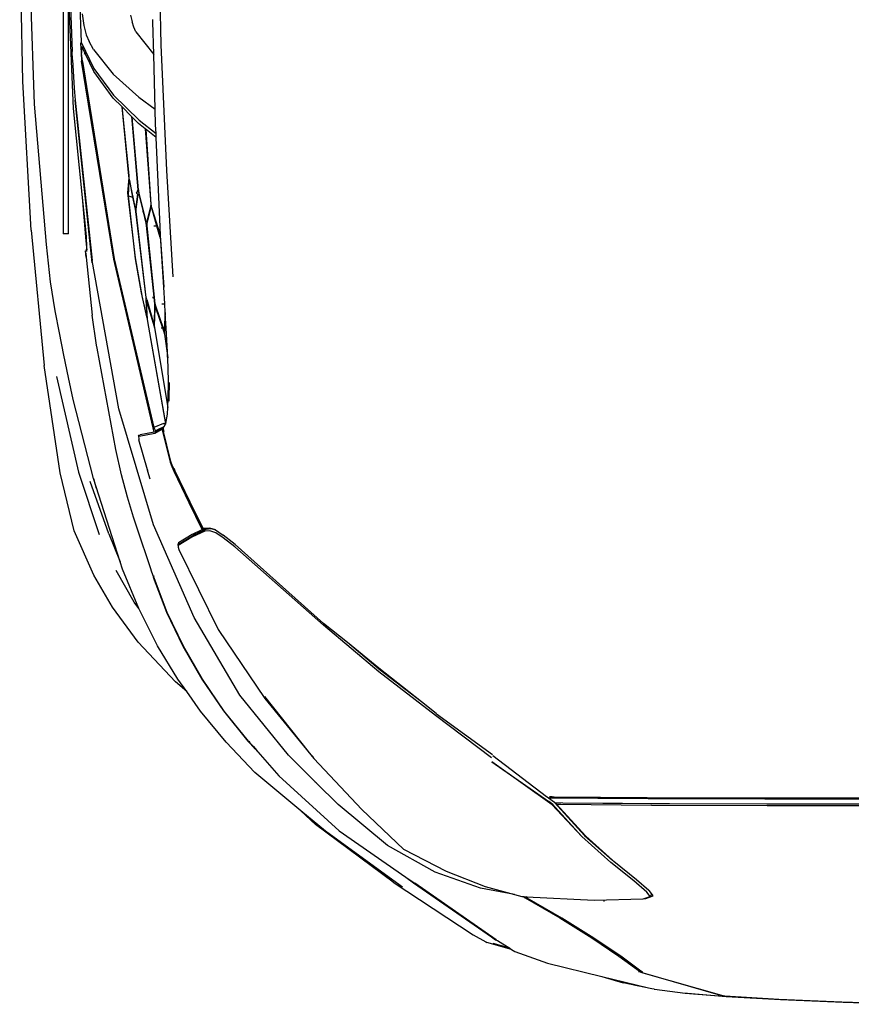
# Model space of a CAD drawing. Units: inches. Extents: x 22042254 to 25404563, y 17568978 to 17626777.
# Tile 10 of 45: x 22042340.5158 to 22042340.9417, y 17568977.6618 to 17568978.1657. Entities that reach past the tile are written whole.
import ezdxf

# ---------------------------------------------------------------- set-up
doc = ezdxf.new("R2010")
doc.units = ezdxf.units.IN
doc.header["$MEASUREMENT"] = 0
doc.layers.add('A-SITE-VEHI', color=8, linetype='Continuous', lineweight=18)
doc.layers.add('Edges', color=250, linetype='Continuous')

# ---------------------------------------------------------------- blocks, each defined once
blk = doc.blocks.new('Nissan Qashqai pl')
at = {"layer": 'Edges'}
for p, q in [((8.01597, 12.81888), (7.96577, 12.81715)), ((7.96683, 12.81735), (8.01677, 12.81906)), ((7.86763, 12.81233), (7.79979, 12.79282)), ((7.80119, 12.79291), (7.86805, 12.81214)), ((7.83626, 12.80972), (7.86763, 12.81233)), ((7.83812, 12.80996), (7.86997, 12.81262)), ((7.86763, 12.81233), (7.86805, 12.81214)), ((7.86903, 12.81242), (7.86805, 12.81214)), ((7.91369, 12.81497), (7.86903, 12.81242)), ((7.86997, 12.81262), (7.91514, 12.8152)), ((7.96577, 12.81715), (7.91369, 12.81497)), ((7.91514, 12.8152), (7.96683, 12.81735)), ((7.7673, 12.79611), (7.80585, 12.80552)), ((7.80866, 12.80621), (7.78484, 12.80117)), ((7.79357, 12.80288), (7.79772, 12.80375)), ((7.81062, 12.80645), (7.80866, 12.80621)), ((7.81062, 12.80645), (7.81073, 12.80648)), ((7.81073, 12.80648), (7.83626, 12.80972)), ((7.83626, 12.80972), (7.83812, 12.80996)), ((7.72226, 12.78511), (7.7673, 12.79611)), ((7.7673, 12.79611), (7.78484, 12.80117)), ((7.78354, 12.80068), (7.78351, 12.80067)), ((7.78647, 12.80131), (7.78656, 12.80134)), ((7.78138, 12.77913), (7.79909, 12.7923)), ((7.79842, 12.79085), (7.78285, 12.7793)), ((7.79759, 12.79204), (7.79909, 12.7923)), ((7.80074, 12.79258), (7.79842, 12.79085)), ((7.79909, 12.7923), (7.79979, 12.79282)), ((7.79952, 12.79237), (7.80074, 12.79258)), ((7.80119, 12.79291), (7.80074, 12.79258)), ((7.69527, 12.77535), (7.72226, 12.78511)), ((7.75906, 12.76414), (7.78138, 12.77913)), ((7.78285, 12.7793), (7.76061, 12.76436)), ((7.6926, 12.77369), (7.67207, 12.76794)), ((7.69111, 12.77277), (7.67743, 12.76878)), ((7.68089, 12.76644), (7.69111, 12.77277)), ((7.69111, 12.77277), (7.6926, 12.77369)), ((7.6926, 12.77369), (7.69527, 12.77535)), ((7.59458, 12.71797), (7.66077, 12.76166)), ((7.61132, 12.71859), (7.67585, 12.76329)), ((7.67993, 12.76585), (7.61247, 12.71901)), ((7.66077, 12.76166), (7.67122, 12.76746)), ((7.67122, 12.76746), (7.67207, 12.76794)), ((7.67585, 12.76329), (7.67933, 12.76572)), ((7.67933, 12.76572), (7.68018, 12.766)), ((7.67993, 12.76585), (7.68018, 12.766)), ((7.68018, 12.766), (7.68089, 12.76644)), ((7.73247, 12.74757), (7.75906, 12.76414)), ((7.76061, 12.76436), (7.73411, 12.74784)), ((7.70382, 12.731), (7.73247, 12.74757)), ((7.73411, 12.74784), (7.70559, 12.73137)), ((7.69488, 12.72832), (7.70101, 12.73001)), ((7.70101, 12.73001), (7.70235, 12.73008)), ((7.70235, 12.73008), (7.70382, 12.731)), ((7.70235, 12.73008), (7.70343, 12.73013)), ((7.70559, 12.73137), (7.70343, 12.73013)), ((7.70343, 12.73013), (7.70481, 12.7302)), ((7.70481, 12.7302), (7.76082, 12.73292)), ((7.70579, 12.73076), (7.70481, 12.7302)), ((7.76082, 12.73292), (7.80143, 12.73178)), ((7.76878, 12.73282), (7.76885, 12.73399)), ((7.80143, 12.73178), (7.80216, 12.73156)), ((7.80216, 12.73156), (7.80372, 12.73151)), ((7.80216, 12.73156), (7.80721, 12.73004)), ((7.80372, 12.73151), (7.80956, 12.72941)), ((7.80721, 12.73004), (7.80447, 12.72626)), ((7.80956, 12.72941), (7.80665, 12.72539)), ((7.80721, 12.73004), (7.80867, 12.72831)), ((7.60245, 12.72211), (7.53868, 12.67594)), ((7.66697, 12.723), (7.62951, 12.70974)), ((7.63858, 12.70891), (7.67084, 12.72167)), ((7.69488, 12.72832), (7.66697, 12.723)), ((7.67084, 12.72167), (7.69488, 12.72832)), ((7.80447, 12.72626), (7.79381, 12.71706)), ((7.80619, 12.725), (7.79586, 12.71608)), ((7.80619, 12.725), (7.80867, 12.72831)), ((7.80665, 12.72539), (7.80619, 12.725)), ((7.59458, 12.71797), (7.53043, 12.67044)), ((7.55011, 12.67573), (7.60515, 12.71393)), ((7.60515, 12.71393), (7.61132, 12.71859)), ((7.60515, 12.71393), (7.61111, 12.71807)), ((7.61183, 12.71862), (7.61111, 12.71807)), ((7.61247, 12.71901), (7.61183, 12.71862)), ((7.79381, 12.71706), (7.77477, 12.70185)), ((7.79586, 12.71608), (7.77724, 12.70105)), ((7.62951, 12.70974), (7.58999, 12.68766)), ((7.60319, 12.69082), (7.63858, 12.70891)), ((7.77477, 12.70185), (7.75074, 12.68033)), ((7.75301, 12.67941), (7.77596, 12.69989)), ((7.77596, 12.69989), (7.75388, 12.67998)), ((7.77724, 12.70105), (7.77596, 12.69989)), ((7.56866, 12.65792), (7.60319, 12.69082)), ((7.58999, 12.68766), (7.5492, 12.654)), ((7.72614, 12.65431), (7.75074, 12.68033)), ((7.75074, 12.68033), (7.72856, 12.65607)), ((7.55011, 12.67573), (7.50008, 12.63025)), ((7.53868, 12.67594), (7.5184, 12.65911)), ((7.75301, 12.67941), (7.72807, 12.65235)), ((7.75388, 12.67998), (7.73238, 12.65652)), ((7.5184, 12.65911), (7.53043, 12.67044)), ((7.5184, 12.65911), (7.48015, 12.62736)), ((7.52891, 12.61585), (7.56866, 12.65792)), ((7.72856, 12.65607), (7.72667, 12.65393)), ((7.73238, 12.65652), (7.72986, 12.65372)), ((7.5492, 12.654), (7.53101, 12.63591)), ((7.72614, 12.65431), (7.67617, 12.61859)), ((7.67617, 12.61859), (7.72327, 12.65136)), ((7.7215, 12.64734), (7.72214, 12.64782)), ((7.72318, 12.64862), (7.72214, 12.64782)), ((7.72807, 12.65235), (7.72318, 12.64862)), ((7.72455, 12.64863), (7.72318, 12.64862)), ((7.72667, 12.65393), (7.72327, 12.65136)), ((7.72606, 12.64765), (7.72382, 12.64759)), ((7.72942, 12.64868), (7.72455, 12.64863)), ((7.72785, 12.6477), (7.72606, 12.64765)), ((7.80482, 12.64828), (7.72785, 12.6477)), ((7.72986, 12.65372), (7.72807, 12.65235)), ((7.72807, 12.65235), (7.73491, 12.65241)), ((7.73098, 12.64869), (7.72942, 12.64868)), ((7.72986, 12.65372), (7.73345, 12.65375)), ((7.76399, 12.64888), (7.73098, 12.64869)), ((7.73345, 12.65375), (7.80829, 12.65437)), ((7.73491, 12.65241), (7.76799, 12.65269)), ((7.76622, 12.64889), (7.76399, 12.64888)), ((7.78115, 12.64897), (7.76622, 12.64889)), ((7.76799, 12.65269), (7.76925, 12.6527)), ((7.76925, 12.6527), (7.78439, 12.65283)), ((7.78224, 12.64898), (7.78115, 12.64897)), ((7.80566, 12.64911), (7.78224, 12.64898)), ((7.78439, 12.65283), (7.80777, 12.65303)), ((7.90142, 12.64867), (7.80482, 12.64828)), ((7.82329, 12.64918), (7.80566, 12.64911)), ((7.80777, 12.65303), (7.82329, 12.65309)), ((7.80829, 12.65437), (7.90396, 12.65472)), ((7.82329, 12.65309), (7.90357, 12.65342)), ((7.90204, 12.64948), (7.82329, 12.64918)), ((8.02732, 12.64849), (7.90142, 12.64867)), ((8.02749, 12.64934), (7.90204, 12.64948)), ((7.90357, 12.65342), (8.0275, 12.6533)), ((7.90396, 12.65472), (8.02759, 12.65454)), ((7.67714, 12.61347), (7.7215, 12.64734)), ((7.53101, 12.63591), (7.50805, 12.61306)), ((7.53101, 12.63591), (7.53009, 12.6353)), ((7.48015, 12.62736), (7.45654, 12.6023)), ((7.48274, 12.61035), (7.50008, 12.63025)), ((7.48836, 12.56635), (7.52891, 12.61585)), ((7.67598, 12.61523), (7.6296, 12.58026)), ((7.50805, 12.61306), (7.46788, 12.56344)), ((7.47438, 12.60148), (7.48041, 12.60787)), ((7.48041, 12.60787), (7.47799, 12.6049)), ((7.47901, 12.60607), (7.4815, 12.60892)), ((7.47901, 12.60607), (7.48009, 12.6074)), ((7.48009, 12.6074), (7.48041, 12.60787)), ((7.48041, 12.60787), (7.48043, 12.60789)), ((7.48043, 12.60789), (7.48069, 12.60817)), ((7.48069, 12.60817), (7.48214, 12.60971)), ((7.4815, 12.60892), (7.48214, 12.60971)), ((7.48214, 12.60971), (7.48274, 12.61035)), ((7.48817, 12.5645), (7.52431, 12.61007)), ((7.52431, 12.61007), (7.52857, 12.61458)), ((7.67691, 12.61295), (7.63059, 12.57913)), ((7.45654, 12.6023), (7.4354, 12.57664)), ((7.45423, 12.57648), (7.47438, 12.60148)), ((7.47504, 12.60161), (7.45491, 12.57668)), ((7.47616, 12.6028), (7.47504, 12.60161)), ((7.47515, 12.60164), (7.47616, 12.6028)), ((7.47616, 12.6028), (7.47799, 12.6049)), ((7.47799, 12.6049), (7.47901, 12.60607)), ((7.4354, 12.57664), (7.42386, 12.56045)), ((7.43626, 12.55019), (7.45423, 12.57648)), ((7.45491, 12.57668), (7.4369, 12.55039)), ((7.6296, 12.58026), (7.58274, 12.54411)), ((7.63007, 12.57872), (7.61803, 12.56913)), ((7.63059, 12.57913), (7.63007, 12.57872)), ((7.44978, 12.50928), (7.48836, 12.56635)), ((7.61803, 12.56913), (7.58288, 12.54113)), ((7.61803, 12.56913), (7.58398, 12.54289)), ((7.42386, 12.56045), (7.41469, 12.55237)), ((7.42386, 12.56045), (7.41661, 12.55027)), ((7.46788, 12.56344), (7.43015, 12.49926)), ((7.41469, 12.55237), (7.38367, 12.51969)), ((7.41661, 12.55027), (7.39973, 12.5227)), ((7.42053, 12.52292), (7.43626, 12.55019)), ((7.4369, 12.55039), (7.42115, 12.52316)), ((7.58274, 12.54411), (7.53689, 12.50568)), ((7.58398, 12.54289), (7.55683, 12.52012)), ((7.58288, 12.54113), (7.55683, 12.52012)), ((7.38367, 12.51969), (7.36237, 12.49067)), ((7.39973, 12.5227), (7.38446, 12.49246)), ((7.40715, 12.49483), (7.42053, 12.52292)), ((7.42115, 12.52316), (7.40781, 12.49514)), ((7.55683, 12.52012), (7.53708, 12.50419)), ((7.41723, 12.44309), (7.44978, 12.50928)), ((7.53689, 12.50568), (7.46355, 12.44079)), ((7.46382, 12.43903), (7.53708, 12.50419)), ((7.39621, 12.46602), (7.40715, 12.49483)), ((7.43015, 12.49926), (7.39627, 12.4227)), ((7.40781, 12.49514), (7.39687, 12.46646)), ((7.36237, 12.49067), (7.34698, 12.4644)), ((7.38053, 12.48658), (7.36552, 12.46044)), ((7.38426, 12.49197), (7.37074, 12.45925)), ((7.38426, 12.49197), (7.38053, 12.48658)), ((7.38446, 12.49246), (7.38426, 12.49197)), ((7.34698, 12.4644), (7.3309, 12.42757)), ((7.39513, 12.46199), (7.39379, 12.45826)), ((7.39648, 12.46548), (7.39513, 12.46199)), ((7.39648, 12.46548), (7.39621, 12.46602)), ((7.39687, 12.46646), (7.39648, 12.46548)), ((7.39676, 12.46492), (7.39668, 12.46506)), ((7.3688, 12.45323), (7.34671, 12.38455)), ((7.35959, 12.43024), (7.3688, 12.45323)), ((7.37074, 12.45925), (7.3688, 12.45323)), ((7.39247, 12.45422), (7.38454, 12.43058)), ((7.39379, 12.45826), (7.39247, 12.45422)), ((7.41665, 12.43928), (7.41687, 12.44057)), ((7.41665, 12.43928), (7.41716, 12.43948)), ((7.41697, 12.43768), (7.41665, 12.43928)), ((7.41686, 12.44121), (7.41723, 12.44309)), ((7.41687, 12.44057), (7.41686, 12.44121)), ((7.41687, 12.44057), (7.41717, 12.44232)), ((7.41689, 12.43978), (7.41687, 12.44057)), ((7.42821, 12.43284), (7.41689, 12.43978)), ((7.41716, 12.43948), (7.41689, 12.43978)), ((7.42833, 12.4307), (7.41697, 12.43768)), ((7.4183, 12.4382), (7.41716, 12.43948)), ((7.41717, 12.44232), (7.41744, 12.44287)), ((7.41747, 12.44292), (7.41744, 12.44287)), ((7.4183, 12.4382), (7.42961, 12.43124)), ((7.46355, 12.44079), (7.4541, 12.43335)), ((7.46382, 12.43903), (7.45415, 12.43132)), ((7.33449, 12.37926), (7.3514, 12.43082)), ((7.35959, 12.43024), (7.34401, 12.38695)), ((7.38454, 12.43058), (7.37986, 12.41639)), ((7.43873, 12.42797), (7.42821, 12.43284)), ((7.43587, 12.42718), (7.42833, 12.4307)), ((7.43832, 12.42716), (7.42961, 12.43124)), ((7.44309, 12.42761), (7.43873, 12.42797)), ((7.44789, 12.42929), (7.44309, 12.42761)), ((7.44771, 12.42699), (7.45415, 12.43132)), ((7.4541, 12.43335), (7.44789, 12.42929)), ((7.3309, 12.42757), (7.31925, 12.37966)), ((7.39627, 12.4227), (7.36761, 12.32692)), ((7.42553, 12.40435), (7.43673, 12.42678)), ((7.43648, 12.4235), (7.42672, 12.4041)), ((7.43673, 12.42678), (7.43587, 12.42718)), ((7.43651, 12.42353), (7.43648, 12.4235)), ((7.43782, 12.42614), (7.43651, 12.42353)), ((7.43673, 12.42678), (7.43832, 12.42716)), ((7.43787, 12.42625), (7.43782, 12.42614)), ((7.43787, 12.42625), (7.43832, 12.42716)), ((7.43787, 12.42625), (7.4389, 12.42689)), ((7.43844, 12.42599), (7.43787, 12.42625)), ((7.43844, 12.42599), (7.43799, 12.42508)), ((7.43832, 12.42716), (7.4389, 12.42689)), ((7.4389, 12.42689), (7.43844, 12.42599)), ((7.43873, 12.42586), (7.43844, 12.42599)), ((7.44298, 12.42535), (7.43873, 12.42586)), ((7.44004, 12.42635), (7.4389, 12.42689)), ((7.44004, 12.42635), (7.44418, 12.42585)), ((7.44771, 12.42699), (7.44298, 12.42535)), ((7.44418, 12.42585), (7.44771, 12.42699)), ((7.37986, 12.41639), (7.375, 12.39997)), ((7.41315, 12.3783), (7.42553, 12.40435)), ((7.42672, 12.4041), (7.41393, 12.37779)), ((7.375, 12.39997), (7.36995, 12.3813)), ((7.34671, 12.38455), (7.34891, 12.39245)), ((7.31925, 12.37966), (7.3059, 12.29098)), ((7.31612, 12.30008), (7.33449, 12.37926)), ((7.34671, 12.38455), (7.32996, 12.31924)), ((7.36995, 12.3813), (7.36534, 12.36039)), ((7.39248, 12.38132), (7.39136, 12.37745)), ((7.39374, 12.38511), (7.39248, 12.38132)), ((7.39133, 12.37737), (7.38437, 12.35258)), ((7.39133, 12.37737), (7.39136, 12.37745)), ((7.40326, 12.3435), (7.41007, 12.37083)), ((7.41007, 12.37083), (7.41147, 12.37465)), ((7.41219, 12.37416), (7.41077, 12.37034)), ((7.41147, 12.37465), (7.41315, 12.3783)), ((7.41393, 12.37779), (7.41219, 12.37416)), ((7.41334, 12.37586), (7.41416, 12.37763)), ((7.41077, 12.37034), (7.40418, 12.34346)), ((7.36534, 12.36039), (7.3497, 12.27675)), ((7.38412, 12.34854), (7.38437, 12.35258)), ((7.38458, 12.34953), (7.38412, 12.34854)), ((7.38412, 12.34854), (7.38529, 12.34833)), ((7.38458, 12.34953), (7.39764, 12.34702)), ((7.39705, 12.34608), (7.38529, 12.34833)), ((7.39764, 12.34702), (7.40264, 12.34394)), ((7.39705, 12.34608), (7.36347, 12.20326)), ((7.36397, 12.20287), (7.39678, 12.34241)), ((7.39156, 12.25473), (7.40622, 12.33886)), ((7.40648, 12.33918), (7.39169, 12.25467)), ((7.39678, 12.34241), (7.39804, 12.34491)), ((7.40464, 12.33886), (7.39678, 12.34241)), ((7.39833, 12.34584), (7.39705, 12.34608)), ((7.39804, 12.34491), (7.39989, 12.34404)), ((7.39804, 12.34491), (7.4012, 12.34407)), ((7.4012, 12.34407), (7.39833, 12.34584)), ((7.39989, 12.34404), (7.40511, 12.34151)), ((7.39989, 12.34404), (7.40478, 12.34174)), ((7.40335, 12.34275), (7.4012, 12.34407)), ((7.4012, 12.34407), (7.40147, 12.344)), ((7.40147, 12.344), (7.40276, 12.34374)), ((7.40264, 12.34394), (7.40326, 12.3435)), ((7.40326, 12.3435), (7.40417, 12.34217)), ((7.40417, 12.34217), (7.40335, 12.34275)), ((7.40418, 12.34346), (7.40405, 12.34294)), ((7.40405, 12.34294), (7.40431, 12.34276)), ((7.40405, 12.34294), (7.40425, 12.34252)), ((7.40411, 12.34347), (7.40418, 12.34346)), ((7.40417, 12.34217), (7.40425, 12.34252)), ((7.40443, 12.34217), (7.40417, 12.34217)), ((7.40418, 12.34346), (7.40447, 12.3434)), ((7.40425, 12.34252), (7.40431, 12.34276)), ((7.40425, 12.34252), (7.40443, 12.34217)), ((7.40431, 12.34276), (7.40447, 12.3434)), ((7.40431, 12.34276), (7.40461, 12.34255)), ((7.40443, 12.34217), (7.40456, 12.34189)), ((7.40463, 12.34217), (7.40443, 12.34217)), ((7.40447, 12.3434), (7.40502, 12.34562)), ((7.40447, 12.3434), (7.4048, 12.34334)), ((7.40463, 12.34217), (7.40456, 12.34189)), ((7.40456, 12.34189), (7.40497, 12.34189)), ((7.40478, 12.34174), (7.40456, 12.34189)), ((7.40461, 12.34255), (7.40469, 12.3424)), ((7.40469, 12.3424), (7.40463, 12.34217)), ((7.40482, 12.34217), (7.40463, 12.34217)), ((7.40464, 12.33886), (7.40622, 12.33886)), ((7.40469, 12.3424), (7.40482, 12.34217)), ((7.40478, 12.34174), (7.40515, 12.34156)), ((7.40511, 12.34151), (7.40478, 12.34174)), ((7.40482, 12.34217), (7.40497, 12.34189)), ((7.40497, 12.34189), (7.40515, 12.34156)), ((7.40511, 12.34151), (7.40521, 12.34146)), ((7.40515, 12.34156), (7.40521, 12.34146)), ((7.40521, 12.34146), (7.40632, 12.33946)), ((7.40622, 12.33886), (7.40632, 12.33946)), ((7.40632, 12.33946), (7.40648, 12.33918)), ((7.40648, 12.33918), (7.4066, 12.33895)), ((7.4066, 12.33895), (7.40795, 12.33127)), ((7.40795, 12.33127), (7.40828, 12.32581)), ((7.36761, 12.32692), (7.34554, 12.2042)), ((7.39714, 12.25992), (7.40828, 12.32581)), ((7.40836, 12.3244), (7.39747, 12.25989)), ((7.40828, 12.32581), (7.40836, 12.3244)), ((7.40836, 12.3244), (7.40865, 12.31952)), ((7.32996, 12.31924), (7.3261, 12.30088)), ((7.40865, 12.31952), (7.40871, 12.30369)), ((7.40921, 12.31837), (7.40908, 12.32063)), ((7.40923, 12.30498), (7.40921, 12.31837)), ((7.3261, 12.30088), (7.32232, 12.28252)), ((7.40871, 12.30369), (7.40814, 12.28481)), ((7.29513, 12.17908), (7.3059, 12.29098)), ((7.32232, 12.28252), (7.3186, 12.26414)), ((7.40539, 12.2651), (7.40814, 12.28481)), ((7.40811, 12.28378), (7.40791, 12.2798)), ((7.40814, 12.28481), (7.40811, 12.28378)), ((7.34938, 12.27412), (7.34574, 12.2495)), ((7.34978, 12.2768), (7.34938, 12.27412)), ((7.3497, 12.27675), (7.34938, 12.27412)), ((7.40791, 12.2798), (7.40588, 12.26512)), ((7.40791, 12.2798), (7.40687, 12.2598)), ((7.40488, 12.26309), (7.40539, 12.2651)), ((7.40588, 12.26512), (7.40585, 12.26319)), ((7.3186, 12.26414), (7.31494, 12.24575)), ((7.39095, 12.23871), (7.39668, 12.25792)), ((7.39691, 12.257), (7.39654, 12.25604)), ((7.39668, 12.25792), (7.39714, 12.25992)), ((7.39684, 12.25593), (7.39691, 12.257)), ((7.39747, 12.25989), (7.39733, 12.25795)), ((7.39733, 12.25795), (7.39774, 12.24387)), ((7.40485, 12.26124), (7.39823, 12.24191)), ((7.39827, 12.24398), (7.40376, 12.25987)), ((7.40279, 12.25987), (7.40376, 12.25987)), ((7.40376, 12.25987), (7.40488, 12.26309)), ((7.40532, 12.26222), (7.40485, 12.26124)), ((7.40532, 12.26117), (7.40532, 12.26222)), ((7.40611, 12.24728), (7.40532, 12.26117)), ((7.40592, 12.26183), (7.40555, 12.26207)), ((7.40585, 12.26319), (7.40592, 12.26183)), ((7.40592, 12.26183), (7.40642, 12.25231)), ((7.40687, 12.2598), (7.40642, 12.25231)), ((7.3407, 12.2016), (7.34574, 12.2495)), ((7.39089, 12.25084), (7.38644, 12.23105)), ((7.3869, 12.23473), (7.39116, 12.25274)), ((7.39012, 12.23681), (7.39099, 12.25068)), ((7.39141, 12.25272), (7.39058, 12.23864)), ((7.3908, 12.23661), (7.39654, 12.25604)), ((7.39114, 12.25178), (7.39089, 12.25084)), ((7.39099, 12.25068), (7.39114, 12.25178)), ((7.39121, 12.25173), (7.39114, 12.25178)), ((7.39116, 12.25274), (7.39156, 12.25473)), ((7.39169, 12.25467), (7.39141, 12.25272)), ((7.39722, 12.24205), (7.39684, 12.25593)), ((7.40642, 12.25231), (7.40611, 12.24728)), ((7.31494, 12.24575), (7.31133, 12.22174)), ((7.39715, 12.24), (7.39722, 12.24205)), ((7.39823, 12.24191), (7.39768, 12.23999)), ((7.39774, 12.24387), (7.39795, 12.24289)), ((7.39795, 12.24289), (7.39827, 12.24398)), ((7.40611, 12.2472), (7.40567, 12.23998)), ((7.40611, 12.2472), (7.40611, 12.24728)), ((7.38128, 12.20212), (7.3869, 12.23473)), ((7.38152, 12.16381), (7.38995, 12.23475)), ((7.39032, 12.23471), (7.38195, 12.16385)), ((7.38995, 12.23475), (7.39012, 12.23681)), ((7.3908, 12.23661), (7.39032, 12.23471)), ((7.39046, 12.17543), (7.3966, 12.23466)), ((7.39058, 12.23864), (7.39067, 12.23763)), ((7.39067, 12.23763), (7.39095, 12.23871)), ((7.39768, 12.23999), (7.39107, 12.17551)), ((7.39566, 12.23466), (7.3966, 12.23466)), ((7.3957, 12.2348), (7.39661, 12.2348)), ((7.3966, 12.23466), (7.39661, 12.2348)), ((7.39661, 12.2348), (7.39715, 12.24)), ((7.40319, 12.23998), (7.40567, 12.23998)), ((7.40567, 12.23998), (7.40484, 12.22617)), ((7.38644, 12.23105), (7.38154, 12.2029)), ((7.40216, 12.18704), (7.40484, 12.22617)), ((7.40484, 12.22617), (7.40226, 12.1836)), ((7.31133, 12.22174), (7.30777, 12.19099)), ((7.40723, 12.12993), (7.41241, 12.21762)), ((7.34554, 12.20616), (7.33168, 12.07174)), ((7.33168, 12.07174), (7.34554, 12.2042)), ((7.3407, 12.2016), (7.34004, 12.19617)), ((7.34033, 12.19813), (7.3407, 12.2016)), ((7.36347, 12.20326), (7.34048, 12.06162)), ((7.34263, 12.07068), (7.36397, 12.20287)), ((7.37498, 12.14844), (7.38128, 12.20212)), ((7.38154, 12.2029), (7.37562, 12.1509)), ((7.34004, 12.19617), (7.34009, 12.19616)), ((7.34009, 12.19616), (7.34097, 12.1962)), ((7.34131, 12.19329), (7.34072, 12.18787)), ((7.34097, 12.1962), (7.341, 12.1962)), ((7.34097, 12.1962), (7.34131, 12.19329)), ((7.34133, 12.19308), (7.34097, 12.18475)), ((7.341, 12.1962), (7.34144, 12.1962)), ((7.34145, 12.19617), (7.341, 12.1962)), ((7.34154, 12.19537), (7.34131, 12.19329)), ((7.34131, 12.19329), (7.34133, 12.19308)), ((7.30777, 12.19099), (7.29801, 12.07497)), ((7.34072, 12.18787), (7.33778, 12.15206)), ((7.34097, 12.18475), (7.33996, 12.17312)), ((7.39898, 12.17558), (7.4017, 12.185)), ((7.4017, 12.185), (7.40216, 12.18704)), ((7.40226, 12.1836), (7.40182, 12.17639)), ((7.40226, 12.1836), (7.40207, 12.18329)), ((7.29513, 12.17908), (7.28835, 12.05625)), ((7.32607, 12.18208), (7.32157, 12.18208)), ((7.32157, 11.66208), (7.32157, 12.18208)), ((7.32607, 12.18208), (7.32607, 11.97794)), ((7.39008, 12.17342), (7.39046, 12.17543)), ((7.39107, 12.17551), (7.39127, 12.17366)), ((7.39494, 12.16159), (7.39898, 12.17558)), ((7.40207, 12.18329), (7.39509, 12.16063)), ((7.39666, 12.17558), (7.39898, 12.17558)), ((7.40182, 12.17639), (7.39862, 12.10249)), ((7.33996, 12.17312), (7.33778, 12.15206)), ((7.39028, 12.17165), (7.38438, 12.14787)), ((7.38773, 12.16389), (7.39008, 12.17342)), ((7.39074, 12.17265), (7.39028, 12.17165)), ((7.39087, 12.17164), (7.39074, 12.17265)), ((7.39387, 12.15956), (7.39087, 12.17164)), ((7.39127, 12.17366), (7.39425, 12.16142)), ((7.38127, 12.15992), (7.37634, 12.13606)), ((7.37916, 12.15176), (7.38118, 12.1619)), ((7.38118, 12.1619), (7.38152, 12.16381)), ((7.38146, 12.16096), (7.38127, 12.15992)), ((7.3817, 12.16004), (7.38146, 12.16096)), ((7.38322, 12.1493), (7.3817, 12.16004)), ((7.38195, 12.16385), (7.38202, 12.1619)), ((7.38202, 12.1619), (7.38379, 12.14973)), ((7.38426, 12.14979), (7.38773, 12.16389)), ((7.38773, 12.16389), (7.38737, 12.16389)), ((7.39414, 12.15763), (7.39387, 12.15956)), ((7.39425, 12.16142), (7.39471, 12.16054)), ((7.39509, 12.16063), (7.39449, 12.15768)), ((7.39471, 12.16054), (7.39494, 12.16159)), ((7.33778, 12.15206), (7.33017, 12.07853)), ((7.37562, 12.1509), (7.37916, 12.15176)), ((7.37642, 12.13802), (7.37916, 12.15176)), ((7.38964, 12.09538), (7.39414, 12.15763)), ((7.39449, 12.15768), (7.39027, 12.09589)), ((7.37596, 12.13603), (7.37498, 12.14844)), ((7.37562, 12.1509), (7.37623, 12.13799)), ((7.37826, 12.0852), (7.38357, 12.14586)), ((7.38403, 12.14592), (7.37876, 12.0857)), ((7.38322, 12.1493), (7.38243, 12.1487)), ((7.38243, 12.1487), (7.38324, 12.14918)), ((7.38357, 12.14586), (7.38243, 12.1487)), ((7.38243, 12.1487), (7.3835, 12.14683)), ((7.38379, 12.14973), (7.38322, 12.1493)), ((7.38324, 12.14918), (7.38322, 12.1493)), ((7.38324, 12.14918), (7.38374, 12.14948)), ((7.38357, 12.14586), (7.3835, 12.14683)), ((7.3835, 12.14683), (7.38403, 12.14592)), ((7.38374, 12.14948), (7.38426, 12.14979)), ((7.38374, 12.14948), (7.38379, 12.14973)), ((7.38403, 12.14592), (7.38424, 12.1495)), ((7.38438, 12.14787), (7.38403, 12.14592)), ((7.38424, 12.1495), (7.38426, 12.14979)), ((7.38427, 12.14952), (7.38424, 12.1495)), ((7.37589, 12.1341), (7.37596, 12.13603)), ((7.37634, 12.13606), (7.37608, 12.13413)), ((7.37623, 12.13799), (7.37624, 12.13703)), ((7.37624, 12.13703), (7.37642, 12.13802)), ((7.37638, 12.13711), (7.37624, 12.13703)), ((7.37008, 12.07708), (7.37589, 12.1341)), ((7.37608, 12.13413), (7.37036, 12.07735)), ((7.40245, 12.02601), (7.40723, 12.12993)), ((7.39862, 12.10249), (7.39027, 12.09589)), ((7.39862, 12.10249), (7.39848, 12.09934)), ((7.38964, 12.09538), (7.38409, 12.09099)), ((7.38449, 12.08832), (7.39848, 12.09934)), ((7.39027, 12.09589), (7.38964, 12.09538)), ((7.39848, 12.09934), (7.39816, 12.09205)), ((7.36331, 12.06744), (7.38449, 12.08832)), ((7.38409, 12.09099), (7.37876, 12.0857)), ((7.39816, 12.09205), (7.39782, 12.07909)), ((7.33017, 12.07853), (7.32607, 11.97794)), ((7.37826, 12.0852), (7.37036, 12.07735)), ((7.37876, 12.0857), (7.37826, 12.0852)), ((7.38423, 12.06929), (7.39782, 12.07909)), ((7.39782, 12.07909), (7.3966, 12.03384)), ((7.29801, 12.07497), (7.29279, 11.92208)), ((7.33087, 12.06192), (7.33168, 12.07174)), ((7.34104, 12.06045), (7.34263, 12.07068)), ((7.36309, 12.07013), (7.34693, 12.0481)), ((7.37008, 12.07708), (7.36309, 12.07013)), ((7.37036, 12.07735), (7.37008, 12.07708)), ((7.32941, 12.03847), (7.33087, 12.06192)), ((7.34048, 12.06162), (7.33691, 12.03944)), ((7.34711, 12.04544), (7.36331, 12.06744)), ((7.36303, 12.05012), (7.38423, 12.06929)), ((7.28835, 12.05625), (7.28572, 11.92208)), ((7.33767, 12.03978), (7.34104, 12.06045)), ((7.33653, 12.02372), (7.34711, 12.04544)), ((7.34693, 12.0481), (7.3402, 12.0337)), ((7.34679, 12.02992), (7.36303, 12.05012)), ((7.32941, 12.03847), (7.32911, 12.03155)), ((7.33645, 12.03215), (7.33691, 12.03944)), ((7.33767, 12.03978), (7.33691, 12.03284)), ((7.32507, 11.92208), (7.32911, 12.03155)), ((7.33615, 12.02477), (7.33645, 12.03215)), ((7.33686, 12.0287), (7.33691, 12.03284)), ((7.33805, 12.02908), (7.33686, 12.0287)), ((7.33805, 12.02908), (7.33737, 12.02763)), ((7.3402, 12.0337), (7.33805, 12.02908)), ((7.33873, 12.03324), (7.3402, 12.0337)), ((7.34679, 12.02992), (7.34316, 12.02313)), ((7.38184, 12.0151), (7.3966, 12.03384)), ((7.3966, 12.03384), (7.39589, 12.00706)), ((7.33294, 11.92208), (7.33653, 12.02372)), ((7.33615, 12.02477), (7.33659, 12.02464)), ((7.33653, 12.02372), (7.33615, 12.02477)), ((7.33737, 12.02763), (7.33686, 12.0287)), ((7.3407, 12.01758), (7.34316, 12.02313)), ((7.40018, 11.92208), (7.40245, 12.02601)), ((7.33865, 12.00996), (7.3407, 12.01758)), ((7.38184, 12.0151), (7.38014, 12.01146)), ((7.33733, 12.00038), (7.33865, 12.00996)), ((7.37751, 12.0015), (7.37864, 12.00699)), ((7.38014, 12.01146), (7.37864, 12.00699)), ((7.39589, 12.00706), (7.39588, 12.00508))]:
    blk.add_line(p, q, dxfattribs=at)
blk = doc.blocks.new('CAR')
blk.add_blockref('Nissan Qashqai pl', (-9.74328, -11.91512))

msp = doc.modelspace()

# ---------------------------------------------------------------- block references
at = {"layer": 'A-SITE-VEHI', "xscale": -0.6191396643141144, "yscale": 0.6191396643141144, "zscale": 0.6191396643141144, "rotation": 180}
msp.add_blockref('CAR', (22042342.03736, 17568978.22147), dxfattribs=at)

doc.saveas('drawing.dxf')
